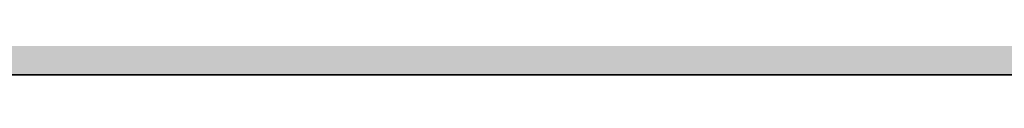
# Model space of a CAD drawing. Units: inches. Extents: x 2083 to 3317, y 1141 to 2115.
# Tile 127 of 256: x 3119.674 to 3123.979, y 1263.261 to 1263.355. Entities that reach past the tile are written whole.
import ezdxf

# ---------------------------------------------------------------- set-up
doc = ezdxf.new("R2010")
doc.units = ezdxf.units.IN
doc.layers.add('A-ANNO-DIMS', color=2, linetype='Continuous', lineweight=18)
doc.layers.add('A-WALL', color=7, linetype='Continuous', lineweight=35)
doc.layers.add('A-WALL-PATT', color=251, linetype='Continuous', lineweight=13, true_color=0x636466)
doc.styles.get("Standard").update_dxf_attribs({"font": 'arial.ttf'})
doc.dimstyles.new('ISO-25', dxfattribs={"dimtxt": 12, "dimasz": 12, "dimexe": 1.25, "dimexo": 0.625, "dimtad": 1, "dimlunit": 3, "dimtxsty": 'Standard', "dimcen": 2.5, "dimadec": 0, "dimazin": 0, "dimtfac": 1, "dimtmove": 0, "dimatfit": 3, "dimfxl": 1, "dimarcsym": 0})

# ---------------------------------------------------------------- blocks, each defined once
blk = doc.blocks.new('*D10')
at = {"layer": 'A-ANNO-DIMS', "color": 0, "lineweight": -2, "transparency": 16777216}
for p, q in [((2862.9598, 1262.6364), (2862.9598, 1201.3844)), ((3126.9598, 1262.6364), (3126.9598, 1201.3844)), ((2874.9598, 1202.6344), (3114.9598, 1202.6344))]:
    blk.add_line(p, q, dxfattribs=at)
at = {"layer": 'A-ANNO-DIMS', "color": 0, "transparency": 16777216}
for points in [[(2874.9598, 1204.6344), (2874.9598, 1200.6344), (2862.9598, 1202.6344)], [(3114.9598, 1204.6344), (3114.9598, 1200.6344), (3126.9598, 1202.6344)]]:
    blk.add_solid(points, dxfattribs=at)
at = {"layer": 'Defpoints', "color": 0, "transparency": 16777216}
for p in [(2862.9598, 1263.2614), (3126.9598, 1263.2614), (3126.9598, 1202.6344)]:
    blk.add_point(p, dxfattribs=at)
at = {"layer": 'A-ANNO-DIMS', "color": 0, "transparency": 16777216, "insert": (2994.9598, 1209.284), "char_height": 12, "attachment_point": 5}
blk.add_mtext("22'", dxfattribs=at)
blk = doc.blocks.new('*D26')
at = {"layer": 'A-ANNO-DIMS', "color": 0, "lineweight": -2, "transparency": 16777216}
for p, q in [((3088.9858, 1274.9151), (3088.9858, 1270.952)), ((3111.24, 1274.9151), (3111.24, 1270.952)), ((3076.9858, 1272.202), (2840.2624, 1272.202)), ((3111.24, 1272.202), (3088.9858, 1272.202)), ((3123.24, 1272.202), (3135.24, 1272.202))]:
    blk.add_line(p, q, dxfattribs=at)
at = {"layer": 'A-ANNO-DIMS', "color": 0, "transparency": 16777216}
for points in [[(3076.9858, 1274.202), (3076.9858, 1270.202), (3088.9858, 1272.202)], [(3123.24, 1274.202), (3123.24, 1270.202), (3111.24, 1272.202)]]:
    blk.add_solid(points, dxfattribs=at)
at = {"layer": 'Defpoints', "color": 0, "transparency": 16777216}
for p in [(3088.9858, 1275.5401), (3111.24, 1275.5401), (3088.9858, 1272.202)]:
    blk.add_point(p, dxfattribs=at)
at = {"layer": 'A-ANNO-DIMS', "color": 0, "transparency": 16777216, "insert": (2952.6241, 1279.0316), "char_height": 12, "attachment_point": 5}
blk.add_mtext('NIGHTSTAND 1\'-10 1/2" TYP.', dxfattribs=at)
blk = doc.blocks.new('*D27')
at = {"layer": 'A-ANNO-DIMS', "color": 0, "lineweight": -2, "transparency": 16777216}
for p, q in [((3114.5782, 1309.7943), (3114.5782, 1321.7943)), ((3111.865, 1297.7943), (3115.8282, 1297.7943)), ((3114.5782, 1297.7943), (3114.5782, 1275.5401)), ((3111.865, 1275.5401), (3115.8282, 1275.5401)), ((3114.5782, 1263.5401), (3114.5782, 1140.9886))]:
    blk.add_line(p, q, dxfattribs=at)
at = {"layer": 'A-ANNO-DIMS', "color": 0, "transparency": 16777216}
for points in [[(3112.5782, 1309.7943), (3116.5782, 1309.7943), (3114.5782, 1297.7943)], [(3112.5782, 1263.5401), (3116.5782, 1263.5401), (3114.5782, 1275.5401)]]:
    blk.add_solid(points, dxfattribs=at)
at = {"layer": 'Defpoints', "color": 0, "transparency": 16777216}
for p in [(3111.24, 1297.7943), (3111.24, 1275.5401), (3114.5782, 1275.5401)]:
    blk.add_point(p, dxfattribs=at)
at = {"layer": 'A-ANNO-DIMS', "color": 0, "transparency": 16777216, "insert": (3107.7485, 1196.2643), "char_height": 12, "attachment_point": 5, "rotation": 90}
blk.add_mtext('1\'-10 1/2" TYP.', dxfattribs=at)

msp = doc.modelspace()

# ---------------------------------------------------------------- hatches: boundary and pattern name
at = {"layer": 'A-WALL-PATT'}
h = msp.add_hatch(color=256, dxfattribs=at)
h.dxf.hatch_style = 1
h.paths.add_polyline_path([(3126.9598, 2020.7614), (2748.9598, 2020.7614), (2604.9598, 2020.7614), (2226.9598, 2020.7614), (2226.9598, 1702.7614), (2466.9598, 1702.7614), (2466.9598, 1582.7614), (2418.9598, 1582.7614), (2418.9598, 1477.7614), (2226.9598, 1477.7614), (2226.9598, 1263.2614), (2544.9598, 1263.2614), (2544.9598, 1411.7614), (2604.9598, 1411.7614), (2685.9598, 1411.7614), (2685.9598, 1420.7614), (2604.9598, 1420.7614), (2604.9598, 1573.7614), (2604.9598, 1702.7614), (2604.9598, 2011.7614), (2748.9598, 2011.7614), (2748.9598, 1702.7614), (2862.9598, 1702.7614), (2862.9598, 1621.7614), (2871.9598, 1621.7614), (2871.9598, 1702.7614), (2883.9598, 1702.7614), (2883.9598, 1706.9395, -0.026459), (2883.9598, 1711.7614), (2757.9598, 1711.7614), (2757.9598, 1807.7614), (2787.9598, 1807.7614), (2787.9598, 1812.2614), (2757.9598, 1812.2614), (2757.9598, 2011.7614), (2877.9598, 2011.7614), (2877.9598, 1812.2614), (2847.9598, 1812.2614), (2847.9598, 1807.7614), (2889.8357, 1807.7614), (2889.8357, 1812.2614), (2882.4598, 1812.2614), (2882.4598, 2011.7614), (3117.9598, 2011.7614), (3117.9598, 1812.2614), (2937.8357, 1812.2614), (2937.8357, 1807.7614), (2995.7098, 1807.7614), (2995.7098, 1796.1177), (3000.2098, 1796.1177), (3000.2098, 1807.7614), (3117.9598, 1807.7614), (3117.9598, 1711.7614), (3000.2098, 1711.7614), (3000.2098, 1760.1177), (2998.5727, 1760.1177, -0.020711), (2995.7098, 1760.1177), (2995.7098, 1711.7614), (2931.9598, 1711.7614), (2931.9598, 1702.7614), (3126.9598, 1702.7614)])
h.paths.add_polyline_path([(2471.4598, 2011.7614), (2471.4598, 1810.0114), (2462.7169, 1810.0114), (2462.7169, 1805.5114), (2505.9598, 1805.5114), (2505.9598, 1810.0114), (2475.9598, 1810.0114), (2475.9598, 2011.7614), (2595.9598, 2011.7614), (2595.9598, 1810.0114), (2565.9598, 1810.0114), (2565.9598, 1805.5114), (2595.9598, 1805.5114), (2595.9598, 1711.7614), (2235.9598, 1711.7614), (2235.9598, 1805.5114), (2353.7098, 1805.5114), (2353.7098, 1796.0542), (2358.2098, 1796.0542), (2358.2098, 1805.5114), (2414.7169, 1805.5114), (2414.7169, 1810.0114), (2235.9598, 1810.0114), (2235.9598, 2011.7614)], flags=16)
h.paths.add_polyline_path([(2270.2047, 1994.61), (2270.2047, 1970.61), (2246.2047, 1970.61), (2246.2047, 1994.61)], flags=0)
edge = h.paths.add_edge_path(flags=0)
edge.add_ellipse((2332.0274, 1899.7982), major_axis=(-3.043, 3.043), ratio=0.168252, start_angle=-161.3322, end_angle=-156.3071, ccw=False)
edge.add_ellipse((2333.082, 1898.7435), major_axis=(-1.0546, 1.0546), ratio=0.453532, start_angle=-123.371, end_angle=-94.1591)
edge = h.paths.add_edge_path(flags=0)
edge.add_ellipse((2332.0274, 1968.8763), major_axis=(3.043, 3.043), ratio=0.168252, start_angle=18.6678, end_angle=23.6929)
edge.add_spline(control_points=[(2332.9256, 1970.6911), (2332.2268, 1970.3361), (2330.8937, 1969.6589), (2328.4131, 1970.9321), (2327.2039, 1967.7487), (2324.7096, 1969.9556), (2322.5328, 1967.0124), (2320.0128, 1971.2958), (2317.6803, 1968.1578), (2316.0405, 1967.102), (2315.4269, 1966.8096)], knot_values=[0, 0, 0, 0, 2.267059, 4.324559, 6.685584, 8.878641, 11.121502, 14.300359, 17.755284, 19.732645, 19.732645, 19.732645, 19.732645], degree=3, periodic=0)
edge.add_ellipse((2332.0274, 1968.8763), major_axis=(3.043, 3.043), ratio=0.168252, start_angle=18.6678, end_angle=23.6929, ccw=False)
edge.add_ellipse((2333.082, 1969.9309), major_axis=(1.0546, 1.0546), ratio=0.453532, start_angle=56.629, end_angle=85.8409, ccw=False)
edge = h.paths.add_edge_path(flags=0)
edge.add_spline(control_points=[(2296.4283, 1967.9879), (2293.6278, 1965.3363), (2287.7036, 1959.7271), (2299.7439, 1949.9957), (2294.5326, 1935.6685), (2290.5732, 1920.6035), (2293.3941, 1909.9737), (2296.1854, 1904.9665)], knot_values=[0.099185, 0.099185, 0.099185, 0.099185, 0.345301, 0.619822, 0.982653, 1.386093, 1.810555, 1.810555, 1.810555, 1.810555], degree=3, periodic=0)
edge.add_spline(control_points=[(2296.1854, 1904.9665), (2297.3836, 1902.6193), (2298.001, 1901.9493), (2298.553, 1901.4682)], knot_values=[0.006246, 0.006246, 0.006246, 0.006246, 0.055476, 0.055476, 0.055476, 0.055476], degree=3, periodic=0)
edge.add_spline(control_points=[(2298.553, 1901.4682), (2297.2586, 1900.9232), (2295.2253, 1900.2321), (2293.0602, 1900.6142), (2292.1014, 1900.7884), (2292.0896, 1900.7906)], knot_values=[0.312835, 0.312835, 0.312835, 0.312835, 0.40178, 0.474987, 0.475903, 0.475903, 0.475903, 0.475903], degree=3, periodic=0)
edge.add_arc((2292.7936, 1904.6641), 3.937, 215.4209, 259.6982, ccw=False)
edge.add_spline(control_points=[(2289.5853, 1902.3823), (2289.4767, 1902.5351), (2289.3685, 1902.688), (2289.2609, 1902.8412)], knot_values=[0.102872, 0.102872, 0.102872, 0.102872, 0.116896, 0.116896, 0.116896, 0.116896], degree=3, periodic=0)
edge.add_spline(control_points=[(2289.2609, 1902.8412), (2288.6866, 1902.5502), (2287.64, 1902.0199), (2285.8813, 1901.874), (2283.853, 1901.5044), (2281.72, 1899.7105), (2278.467, 1899.4929), (2276.1571, 1901.8832), (2272.259, 1899.8041), (2267.7776, 1901.8432), (2262.2439, 1900.184), (2257.4149, 1901.7821), (2254.3184, 1900.7261), (2253.1783, 1900.3373)], knot_values=[0, 0, 0, 0, 1.907977, 3.477176, 5.261074, 7.972851, 11.680248, 13.717921, 16.939592, 22.789562, 27.502503, 33.595215, 37.145618, 37.145618, 37.145618, 37.145618], degree=3, periodic=0)
edge.add_line((2253.1783, 1900.3373), (2250.2442, 1902.8412))
edge.add_line((2250.2442, 1902.8412), (2250.2442, 1965.8333))
edge.add_line((2250.2442, 1965.8333), (2253.1783, 1968.3371))
edge.add_spline(control_points=[(2253.1783, 1968.3371), (2254.3184, 1967.9483), (2257.4149, 1966.8924), (2262.2439, 1968.4904), (2267.7776, 1966.8313), (2271.5267, 1968.5372), (2273.8759, 1967.8283), (2274.2067, 1967.7276)], knot_values=[0, 0, 0, 0, 0.09018, 0.244935, 0.364644, 0.513233, 0.537855, 0.537855, 0.537855, 0.537855], degree=3, periodic=0)
edge.add_arc((2274.3529, 1963.7933), 3.937, 72.0511, 92.1279, ccw=False)
edge.add_arc((2281.2969, 1985.23), 18.5963, 252.05113, 288.56572)
edge.add_arc((2292.3167, 1956.0289), 12.6461, 71.02679, 113.77822, ccw=False)
edge = h.paths.add_edge_path(flags=0)
edge.add_spline(control_points=[(2274.8994, 1951.8562), (2275.0662, 1951.6166), (2275.2327, 1951.3766), (2275.398, 1951.1359)], knot_values=[1.409916, 1.409916, 1.409916, 1.409916, 1.43159, 1.43159, 1.43159, 1.43159], degree=3, periodic=0)
edge.add_spline(control_points=[(2275.398, 1951.1359), (2275.7921, 1950.5619), (2276.1792, 1949.9838), (2276.5455, 1949.3971)], knot_values=[1.358238, 1.358238, 1.358238, 1.358238, 1.409916, 1.409916, 1.409916, 1.409916], degree=3, periodic=0)
edge.add_line((2276.5455, 1949.3971), (2277.4373, 1947.8622))
edge.add_spline(control_points=[(2277.4373, 1947.8622), (2276.3038, 1945.6731), (2274.6397, 1942.4269), (2274.6316, 1938.0939), (2272.7991, 1930.8515), (2274.3564, 1943.897), (2275.9477, 1947.9234), (2276.5455, 1949.3971)], knot_values=[0.005632, 0.005632, 0.005632, 0.005632, 0.186014, 0.266002, 0.357087, 0.59639, 0.739732, 0.739732, 0.739732, 0.739732], degree=3, periodic=0)
edge.add_spline(control_points=[(2276.5455, 1949.3971), (2276.1792, 1949.9838), (2275.7921, 1950.5619), (2275.398, 1951.1359)], knot_values=[1.358238, 1.358238, 1.358238, 1.358238, 1.409916, 1.409916, 1.409916, 1.409916], degree=3, periodic=0)
edge.add_spline(control_points=[(2275.398, 1951.1359), (2274.9425, 1950.0805), (2274.2078, 1948.0253), (2273.9346, 1944.8515), (2272.4685, 1937.6275), (2273.4662, 1945.6965), (2274.7006, 1951.0595), (2274.8994, 1951.8562)], knot_values=[0.104364, 0.104364, 0.104364, 0.104364, 0.189636, 0.269624, 0.36071, 0.600013, 0.644622, 0.644622, 0.644622, 0.644622], degree=3, periodic=0)
h.paths.add_polyline_path([(2269.1675, 1963.1276, -0.357527), (2268.1706, 1960.9764, -0.092561), (2268.1706, 1939.4363, -0.357527), (2269.1675, 1937.2851, -0.357527), (2267.0163, 1938.282, -0.164785), (2254.6856, 1938.282, -0.357527), (2252.5344, 1937.2851, -0.357527), (2253.5313, 1939.4363, -0.092561), (2253.5313, 1960.9764, -0.357527), (2252.5344, 1963.1276, -0.357527), (2254.6856, 1962.1307, -0.164785), (2267.0163, 1962.1307, -0.357527)], flags=0)
h.paths.add_polyline_path([(2248.8741, 1967.8018), (2248.8741, 1957.0277), (2249.4578, 1957.0277), (2249.4578, 1911.6468), (2248.8741, 1911.6468), (2248.8741, 1900.8727), (2246.5119, 1900.8727, 0.197327), (2244.1497, 1902.4569), (2244.1497, 1966.2176, 0.197327), (2246.5119, 1967.8018)], flags=0)
h.paths.add_polyline_path([(2269.1675, 1931.3893, -0.357527), (2268.1706, 1929.2381, -0.092561), (2268.1706, 1907.6981, -0.357527), (2269.1675, 1905.5469, -0.357527), (2267.0163, 1906.5438, -0.164785), (2254.6856, 1906.5438, -0.357527), (2252.5344, 1905.5469, -0.357527), (2253.5313, 1907.6981, -0.092561), (2253.5313, 1929.2381, -0.357527), (2252.5344, 1931.3893, -0.357527), (2254.6856, 1930.3925, -0.164785), (2267.0163, 1930.3925, -0.357527)], flags=0)
edge = h.paths.add_edge_path(flags=0)
edge.add_spline(control_points=[(2276.1969, 1906.7237), (2276.1681, 1909.0289), (2276.114, 1913.3719), (2270.5984, 1924.925), (2273.9052, 1919.0128), (2275.9217, 1916.2621), (2275.4746, 1912.4021), (2277.2579, 1910.3806), (2276.696, 1908.225), (2276.6462, 1906.813), (2276.6178, 1906.0084)], knot_values=[0, 0, 0, 0, 8.61026, 16.221274, 18.843057, 23.804898, 27.440828, 29.356102, 31.203478, 33.650687, 33.650687, 33.650687, 33.650687], degree=3, periodic=0)
edge.add_spline(control_points=[(2276.6178, 1906.0084), (2276.6233, 1905.6241), (2276.4977, 1904.6287), (2275.4418, 1903.8547), (2274.9373, 1903.0804), (2274.8591, 1902.8412)], knot_values=[0.156488, 0.156488, 0.156488, 0.156488, 0.184398, 0.231376, 0.250598, 0.250598, 0.250598, 0.250598], degree=3, periodic=0)
edge.add_line((2274.8591, 1902.8412), (2276.506, 1902.8412))
edge.add_spline(control_points=[(2276.506, 1902.8412), (2276.7883, 1903.0849), (2277.6651, 1904.1252), (2278.2495, 1904.3407), (2277.6539, 1908.5274), (2278.1557, 1906.2278), (2278.1005, 1905.2859), (2278.8467, 1904.069), (2277.8568, 1903.4149), (2277.8742, 1902.991), (2277.9036, 1902.8412)], knot_values=[0.059574, 0.059574, 0.059574, 0.059574, 0.080753, 0.103741, 0.16972, 0.176036, 0.207137, 0.240474, 0.262341, 0.27366, 0.27366, 0.27366, 0.27366], degree=3, periodic=0)
edge.add_line((2277.9036, 1902.8412), (2280.0298, 1902.8412))
edge.add_spline(control_points=[(2280.0298, 1902.8412), (2279.8882, 1903.0884), (2279.4993, 1903.9816), (2280.1523, 1905.9393), (2278.1036, 1909.6578), (2279.7624, 1907.1853), (2280.3279, 1904.8749), (2280.4851, 1903.4896), (2281.4633, 1903.2494), (2281.7583, 1902.9365), (2281.834, 1902.8412)], knot_values=[0.013856, 0.013856, 0.013856, 0.013856, 0.034874, 0.088867, 0.107879, 0.126738, 0.158714, 0.193757, 0.217487, 0.226722, 0.226722, 0.226722, 0.226722], degree=3, periodic=0)
edge.add_spline(control_points=[(2281.834, 1902.8412), (2281.7875, 1902.8267), (2281.647, 1902.783), (2281.3955, 1902.8595), (2281.0881, 1902.9852), (2280.7207, 1903.0609), (2280.3335, 1903.0257), (2280.1248, 1902.8989), (2280.0298, 1902.8412)], knot_values=[0, 0, 0, 0, 0.14413, 0.435517, 0.749276, 1.153046, 1.548371, 1.878348, 1.878348, 1.878348, 1.878348], degree=3, periodic=0)
edge.add_line((2280.0298, 1902.8412), (2277.9036, 1902.8412))
edge.add_spline(control_points=[(2277.9036, 1902.8412), (2277.8929, 1902.7959), (2277.8654, 1902.6796), (2277.6075, 1902.6875), (2277.2741, 1902.8007), (2276.8379, 1902.6198), (2276.5838, 1902.7893), (2276.506, 1902.8412)], knot_values=[0, 0, 0, 0, 0.127189, 0.326199, 0.628009, 1.24357, 1.515331, 1.515331, 1.515331, 1.515331], degree=3, periodic=0)
edge.add_line((2276.506, 1902.8412), (2274.8591, 1902.8412))
edge.add_spline(control_points=[(2274.8591, 1902.8412), (2274.8144, 1902.8986), (2274.7251, 1903.0134), (2274.4935, 1903.119), (2274.2443, 1902.9605), (2273.9371, 1903.1849), (2273.614, 1902.9831), (2273.4083, 1902.883), (2273.3223, 1902.8412)], knot_values=[0, 0, 0, 0, 0.21843, 0.436957, 0.687977, 0.990379, 1.398396, 1.69185, 1.69185, 1.69185, 1.69185], degree=3, periodic=0)
edge.add_spline(control_points=[(2273.3223, 1902.8412), (2273.6167, 1903.4457), (2274.274, 1904.5383), (2276.0272, 1904.5737), (2276.207, 1906.5836), (2276.1969, 1906.7237)], knot_values=[0.012227, 0.012227, 0.012227, 0.012227, 0.059472, 0.106218, 0.134458, 0.134458, 0.134458, 0.134458], degree=3, periodic=0)
h.paths.add_polyline_path([(2270.7761, 1897.7898), (2270.7761, 1873.7898), (2246.7761, 1873.7898), (2246.7761, 1897.7898)], flags=0)
h.paths.add_polyline_path([(2353.7098, 1760.0051), (2353.7098, 1760.0542), (2358.2098, 1760.0542, -0.033729)], flags=0)
h.paths.add_polyline_path([(2321.8191, 1737.5292), (2341.9953, 1737.5292, -0.414214), (2343.2033, 1736.3212), (2343.2033, 1721.0206, -0.414214), (2341.9953, 1719.8127), (2321.8191, 1719.8127, -0.414214), (2320.6112, 1721.0206), (2320.6112, 1736.3212, -0.414214)], flags=0)
h.paths.add_polyline_path([(2324.235, 1736.3212), (2339.5794, 1736.3212, -0.414214), (2341.9953, 1733.9053), (2341.9953, 1725.4497, -0.414214), (2339.5794, 1723.0338), (2333.6806, 1723.0338), (2333.8453, 1722.0455, -0.870646), (2335.4254, 1721.8259, -0.767327), (2333.9227, 1721.4232), (2331.291, 1721.4232, -0.767327), (2329.7883, 1721.8259, -0.870646), (2331.3684, 1722.0455), (2331.5331, 1723.0338), (2324.235, 1723.0338, -0.414214), (2321.8191, 1725.4497), (2321.8191, 1733.9053, -0.414214)], flags=0)
h.paths.add_polyline_path([(2570.4838, 1928.6154), (2589.6838, 1928.6154), (2590.1688, 1928.6154), (2590.1688, 1904.9934), (2570.4838, 1904.9934)], flags=0)
h.paths.add_polyline_path([(2574.4473, 1927.2638, -1), (2572.8288, 1927.2638, -1)], flags=0)
h.paths.add_polyline_path([(2573.0899, 1926.9409), (2573.925, 1927.776), (2574.1477, 1927.5533), (2573.3126, 1926.7182)], flags=0)
h.paths.add_polyline_path([(2578.7791, 1919.7296, -1), (2571.5917, 1919.7296, -1)], flags=0)
h.paths.add_polyline_path([(2578.3854, 1919.7296, -1), (2571.9854, 1919.7296, -1)], flags=0)
h.paths.add_polyline_path([(2331.5958, 1729.4762, -1), (2333.618, 1729.4762, -1)], flags=0)
h.paths.add_polyline_path([(2578.0342, 1927.2638, -1), (2576.4157, 1927.2638, -1)], flags=0)
h.paths.add_polyline_path([(2576.6889, 1927.5311), (2576.9116, 1927.7538), (2577.7467, 1926.9186), (2577.524, 1926.6959)], flags=0)
h.paths.add_polyline_path([(2578.1391, 1909.8595, -1), (2572.2317, 1909.8595, -1)], flags=0)
h.paths.add_polyline_path([(2577.7454, 1909.8595, -1), (2572.6254, 1909.8595, -1)], flags=0)
h.paths.add_polyline_path([(2583.7977, 1927.2638, -1), (2582.1792, 1927.2638, -1)], flags=0)
h.paths.add_polyline_path([(2582.7186, 1927.7538), (2583.5538, 1926.9186), (2583.3311, 1926.6959), (2582.4959, 1927.5311)], flags=0)
h.paths.add_polyline_path([(2582.4959, 1927.5311), (2582.7186, 1927.7538), (2583.5538, 1926.9186), (2583.3311, 1926.6959)], flags=0)
h.paths.add_polyline_path([(2587.7391, 1920.5296, -1), (2581.8317, 1920.5296, -1)], flags=0)
h.paths.add_polyline_path([(2587.3454, 1920.5296, -1), (2582.2254, 1920.5296, -1)], flags=0)
h.paths.add_polyline_path([(2587.3846, 1927.2638, -1), (2585.7661, 1927.2638, -1)], flags=0)
h.paths.add_polyline_path([(2586.082, 1926.9802), (2586.9172, 1927.8154), (2587.1399, 1927.5927), (2586.3047, 1926.7575)], flags=0)
h.paths.add_polyline_path([(2588.3791, 1910.6595, -1), (2581.1917, 1910.6595, -1)], flags=0)
h.paths.add_polyline_path([(2587.9854, 1910.6595, -1), (2581.5854, 1910.6595, -1)], flags=0)
h.paths.add_polyline_path([(2417.1677, 1729.4779), (2437.3439, 1729.4779, -0.414214), (2438.5519, 1728.2699), (2438.5519, 1712.9693, -0.414214), (2437.3439, 1711.7614), (2417.1677, 1711.7614, -0.414214), (2415.9598, 1712.9693), (2415.9598, 1728.2699, -0.414214)], flags=0)
h.paths.add_polyline_path([(2419.5836, 1728.2699), (2434.928, 1728.2699, -0.414214), (2437.3439, 1725.8541), (2437.3439, 1717.3984, -0.414214), (2434.928, 1714.9825), (2429.0292, 1714.9825), (2429.1939, 1713.9942, -0.870646), (2430.774, 1713.7746, -0.767327), (2429.2713, 1713.372), (2426.6396, 1713.372, -0.767327), (2425.1369, 1713.7746, -0.870646), (2426.717, 1713.9942), (2426.8817, 1714.9825), (2419.5836, 1714.9825, -0.414214), (2417.1677, 1717.3984), (2417.1677, 1725.8541, -0.414214)], flags=0)
h.paths.add_polyline_path([(2419.5836, 1728.2699), (2434.928, 1728.2699, -0.414214), (2437.3439, 1725.8541), (2437.3439, 1717.3984, -0.414214), (2434.928, 1714.9825), (2429.0292, 1714.9825), (2428.3581, 1719.009), (2427.5528, 1719.009), (2426.8817, 1714.9825), (2419.5836, 1714.9825, -0.414214), (2417.1677, 1717.3984), (2417.1677, 1725.8541, -0.414214)], flags=0)
h.paths.add_polyline_path([(2426.9444, 1721.4249, -1), (2428.9666, 1721.4249, -1)], flags=0)
h.paths.add_polyline_path([(2475.9598, 1702.7614), (2595.9598, 1702.7614), (2595.9598, 1582.7614), (2475.9598, 1582.7614)], flags=16)
h.paths.add_polyline_path([(2427.9598, 1573.7614), (2595.9598, 1573.7614), (2595.9598, 1468.7614), (2595.9598, 1420.7614), (2384.4598, 1420.7614), (2384.4598, 1468.7614), (2427.9598, 1468.7614)], flags=16)
h.paths.add_polyline_path([(2379.9598, 1468.7614), (2379.9598, 1420.7614), (2235.9598, 1420.7614), (2235.9598, 1468.7614)], flags=16)
h.paths.add_polyline_path([(2317.816, 1466.6958), (2337.9922, 1466.6958, -0.414214), (2339.2002, 1465.4878), (2339.2002, 1450.1872, -0.414214), (2337.9922, 1448.9792), (2317.816, 1448.9792, -0.414214), (2316.6081, 1450.1872), (2316.6081, 1465.4878, -0.414214)], flags=0)
h.paths.add_polyline_path([(2320.2319, 1465.4878), (2335.5763, 1465.4878, -0.414214), (2337.9922, 1463.0719), (2337.9922, 1454.6163, -0.414214), (2335.5763, 1452.2004), (2329.6775, 1452.2004), (2329.8422, 1451.212, -0.870646), (2331.4223, 1450.9925, -0.767327), (2329.9196, 1450.5898), (2327.2879, 1450.5898, -0.767327), (2325.7852, 1450.9925, -0.870646), (2327.3653, 1451.212), (2327.53, 1452.2004), (2320.2319, 1452.2004, -0.414214), (2317.816, 1454.6163), (2317.816, 1463.0719, -0.414214)], flags=0)
h.paths.add_polyline_path([(2320.2319, 1465.4878), (2335.5763, 1465.4878, -0.414214), (2337.9922, 1463.0719), (2337.9922, 1454.6163, -0.414214), (2335.5763, 1452.2004), (2329.6775, 1452.2004), (2329.0064, 1456.2269), (2328.2011, 1456.2269), (2327.53, 1452.2004), (2320.2319, 1452.2004, -0.414214), (2317.816, 1454.6163), (2317.816, 1463.0719, -0.414214)], flags=0)
h.paths.add_polyline_path([(2327.5926, 1458.6428, -1), (2329.6148, 1458.6428, -1)], flags=0)
h.paths.add_polyline_path([(2244.4117, 1433.3405), (2241.9209, 1433.3405, -0.414214), (2240.0179, 1435.2435), (2240.0179, 1440.9528, -0.414211), (2241.9209, 1442.8559), (2244.4117, 1442.8559, -1.976472)], flags=0)
h.paths.add_polyline_path([(2245.3569, 1434.3975, -0.414214), (2245.3569, 1441.7988, -2.144098)], flags=0)
h.paths.add_polyline_path([(2535.9598, 1416.2614), (2535.9598, 1272.2614), (2235.9598, 1272.2614), (2235.9598, 1416.2614)], flags=16)
h.paths.add_polyline_path([(2260.1196, 1384.2928), (2260.1196, 1362.0386), (2237.8654, 1362.0386), (2237.8654, 1384.2928)], flags=0)
edge = h.paths.add_edge_path(flags=0)
edge.add_line((2318.2518, 1362.0933), (2318.1458, 1362.001))
edge.add_ellipse((2317.4451, 1360.431), major_axis=(2.8216, 2.8216), ratio=0.168252, start_angle=18.6678, end_angle=20.9481, ccw=False)
edge.add_ellipse((2318.423, 1361.409), major_axis=(0.9779, 0.9779), ratio=0.453532, start_angle=56.629, end_angle=70.2262, ccw=False)
edge = h.paths.add_edge_path(flags=0)
edge.add_line((2319.1074, 1295.5711), (2319.015, 1295.6771))
edge.add_ellipse((2317.4451, 1296.3778), major_axis=(-2.8216, 2.8216), ratio=0.168252, start_angle=-161.3322, end_angle=-159.0519, ccw=False)
edge.add_ellipse((2318.423, 1295.3999), major_axis=(-0.9779, 0.9779), ratio=0.453532, start_angle=-123.371, end_angle=-109.7738)
edge = h.paths.add_edge_path(flags=0)
edge.add_spline(control_points=[(2284.2103, 1301.1702), (2284.5807, 1300.4447), (2284.8912, 1299.892), (2285.1596, 1299.461)], knot_values=[0.039066, 0.039066, 0.039066, 0.039066, 0.055476, 0.055476, 0.055476, 0.055476], degree=3, periodic=0)
edge.add_line((2285.1596, 1299.461), (2284.2103, 1301.1702))
edge = h.paths.add_edge_path(flags=0)
edge.add_line((2280.4125, 1297.298), (2283.37, 1297.0361))
edge.add_line((2283.37, 1297.0361), (2286.4057, 1297.9263))
edge.add_spline(control_points=[(2286.4057, 1297.9263), (2285.3055, 1297.4631), (2284.3448, 1297.1292), (2283.37, 1297.0361)], knot_values=[0.394369, 0.394369, 0.394369, 0.394369, 0.475903, 0.475903, 0.475903, 0.475903], degree=3, periodic=0)
edge.add_spline(control_points=[(2283.37, 1297.0361), (2283.2814, 1297.0277), (2282.3163, 1296.9573), (2281.3125, 1297.1345), (2280.4234, 1297.296), (2280.4125, 1297.298)], knot_values=[0.312835, 0.312835, 0.312835, 0.312835, 0.320246, 0.393453, 0.394369, 0.394369, 0.394369, 0.394369], degree=3, periodic=0)
edge = h.paths.add_edge_path(flags=0)
edge.add_line((2284.4356, 1359.6073), (2280.4463, 1355.328))
edge.add_line((2280.4463, 1355.328), (2279.58, 1351.0178))
edge.add_line((2279.58, 1351.0178), (2282.413, 1346.5804))
edge.add_spline(control_points=[(2282.413, 1346.5804), (2283.1533, 1345.5892), (2284.2529, 1344.0289), (2284.801, 1342.3872), (2284.9352, 1341.8055)], knot_values=[1.240098, 1.240098, 1.240098, 1.240098, 1.332892, 1.382712, 1.382712, 1.382712, 1.382712], degree=3, periodic=0)
edge.add_spline(control_points=[(2284.9352, 1341.8055), (2285.3191, 1340.1406), (2285.233, 1338.4092), (2284.9099, 1336.6541)], knot_values=[1.097484, 1.097484, 1.097484, 1.097484, 1.240098, 1.240098, 1.240098, 1.240098], degree=3, periodic=0)
edge.add_spline(control_points=[(2284.9099, 1336.6541), (2284.5868, 1334.899), (2284.0267, 1333.1203), (2283.4626, 1331.3606)], knot_values=[0.95487, 0.95487, 0.95487, 0.95487, 1.097484, 1.097484, 1.097484, 1.097484], degree=3, periodic=0)
edge.add_line((2283.4626, 1331.3606), (2281.8904, 1326.1534))
edge.add_line((2281.8904, 1326.1534), (2280.7563, 1321.0561))
edge.add_line((2280.7563, 1321.0561), (2280.2992, 1316.002))
edge.add_line((2280.2992, 1316.002), (2280.7159, 1310.9501))
edge.add_line((2280.7159, 1310.9501), (2282.0281, 1305.9721))
edge.add_line((2282.0281, 1305.9721), (2284.2103, 1301.1702))
edge.add_spline(control_points=[(2284.2103, 1301.1702), (2283.3407, 1302.7302), (2282.6119, 1304.3365), (2282.0281, 1305.9721)], knot_values=[0.099185, 0.099185, 0.099185, 0.099185, 0.241799, 0.241799, 0.241799, 0.241799], degree=3, periodic=0)
edge.add_spline(control_points=[(2282.0281, 1305.9721), (2281.4443, 1307.6078), (2281.0055, 1309.2728), (2280.7159, 1310.9501)], knot_values=[0.241799, 0.241799, 0.241799, 0.241799, 0.384413, 0.384413, 0.384413, 0.384413], degree=3, periodic=0)
edge.add_spline(control_points=[(2280.7159, 1310.9501), (2280.4332, 1312.5876), (2280.2894, 1314.277), (2280.2989, 1315.962), (2280.2992, 1316.002)], knot_values=[0.384413, 0.384413, 0.384413, 0.384413, 0.523647, 0.527028, 0.527028, 0.527028, 0.527028], degree=3, periodic=0)
edge.add_spline(control_points=[(2280.2992, 1316.002), (2280.3123, 1317.687), (2280.4779, 1319.3679), (2280.7563, 1321.0561)], knot_values=[0.527028, 0.527028, 0.527028, 0.527028, 0.669642, 0.669642, 0.669642, 0.669642], degree=3, periodic=0)
edge.add_spline(control_points=[(2280.7563, 1321.0561), (2281.0346, 1322.7443), (2281.4259, 1324.4396), (2281.8904, 1326.1534)], knot_values=[0.669642, 0.669642, 0.669642, 0.669642, 0.812256, 0.812256, 0.812256, 0.812256], degree=3, periodic=0)
edge.add_spline(control_points=[(2281.8904, 1326.1534), (2282.2644, 1327.5333), (2282.7879, 1329.2618), (2283.3528, 1331.0178), (2283.4626, 1331.3606)], knot_values=[0.812256, 0.812256, 0.812256, 0.812256, 0.927087, 0.95487, 0.95487, 0.95487, 0.95487], degree=3, periodic=0)
edge.add_line((2283.4626, 1331.3606), (2284.9099, 1336.6541))
edge.add_line((2284.9099, 1336.6541), (2284.9352, 1341.8055))
edge.add_line((2284.9352, 1341.8055), (2282.413, 1346.5804))
edge.add_spline(control_points=[(2282.413, 1346.5804), (2281.2751, 1348.1038), (2280.0784, 1349.5703), (2279.58, 1351.0178)], knot_values=[1.382712, 1.382712, 1.382712, 1.382712, 1.525326, 1.525326, 1.525326, 1.525326], degree=3, periodic=0)
edge.add_spline(control_points=[(2279.58, 1351.0178), (2279.4433, 1351.4147), (2279.1363, 1352.8569), (2279.7352, 1354.2904), (2280.4463, 1355.328)], knot_values=[1.525326, 1.525326, 1.525326, 1.525326, 1.564439, 1.667941, 1.667941, 1.667941, 1.667941], degree=3, periodic=0)
edge.add_spline(control_points=[(2280.4463, 1355.328), (2281.4261, 1356.7578), (2282.9308, 1358.1826), (2284.4356, 1359.6073)], knot_values=[1.667941, 1.667941, 1.667941, 1.667941, 1.810555, 1.810555, 1.810555, 1.810555], degree=3, periodic=0)
edge.add_arc((2280.6231, 1348.5182), 11.7262, 71.02679, 113.77822)
edge.add_arc((2270.4049, 1375.5952), 17.2436, 252.05113, 288.56572, ccw=False)
edge.add_arc((2263.966, 1355.7178), 3.6506, 72.0511, 92.1279)
edge.add_arc((2263.966, 1355.7178), 3.6506, 92.1279, 177.9851)
edge.add_spline(control_points=[(2260.3176, 1355.8462), (2260.2604, 1354.2207), (2260.5513, 1350.1865), (2262.9993, 1346.7663), (2264.4727, 1344.649)], knot_values=[1.43159, 1.43159, 1.43159, 1.43159, 1.564144, 1.770695, 1.770695, 1.770695, 1.770695], degree=3, periodic=0)
edge.add_line((2264.4727, 1344.649), (2264.9356, 1343.9825))
edge.add_spline(control_points=[(2263.801, 1340.2481), (2263.8432, 1340.5141), (2264.0672, 1341.7565), (2264.5127, 1343.0025), (2264.935, 1343.9811)], knot_values=[0.53657, 0.53657, 0.53657, 0.53657, 0.559349, 0.644622, 0.644622, 0.644622, 0.644622], degree=3, periodic=0)
edge.add_spline(control_points=[(2264.935, 1343.9811), (2265.1178, 1343.715), (2265.2989, 1343.4479), (2265.4768, 1343.1794)], knot_values=[1.384077, 1.384077, 1.384077, 1.384077, 1.409916, 1.409916, 1.409916, 1.409916], degree=3, periodic=0)
edge.add_spline(control_points=[(2265.4768, 1343.1794), (2265.6546, 1342.9108), (2265.8293, 1342.6408), (2265.9991, 1342.3688)], knot_values=[1.358238, 1.358238, 1.358238, 1.358238, 1.384077, 1.384077, 1.384077, 1.384077], degree=3, periodic=0)
edge.add_line((2265.9991, 1342.3688), (2266.826, 1340.9455))
edge.add_spline(control_points=[(2266.826, 1340.9455), (2268.8944, 1337.0897), (2271.3982, 1325.843), (2270.5162, 1310.5686), (2275.9194, 1301.8606), (2277.7895, 1299.1994)], knot_values=[0.116896, 0.116896, 0.116896, 0.116896, 0.472987, 1.050969, 1.313793, 1.313793, 1.313793, 1.313793], degree=3, periodic=0)
edge.add_spline(control_points=[(2277.7895, 1299.1994), (2277.8394, 1299.1285), (2277.8894, 1299.0575), (2277.9396, 1298.9866)], knot_values=[0.109884, 0.109884, 0.109884, 0.109884, 0.116896, 0.116896, 0.116896, 0.116896], degree=3, periodic=0)
edge.add_line((2277.9396, 1298.9866), (2277.7888, 1299.1991))
edge.add_spline(control_points=[(2277.7888, 1299.1991), (2277.2566, 1298.9294), (2276.2864, 1298.4379), (2275.0394, 1298.3344), (2274.3833, 1298.2389), (2274.2153, 1298.2093)], knot_values=[33.12187, 33.12187, 33.12187, 33.12187, 35.029056, 36.598255, 37.144827, 37.144827, 37.144827, 37.144827], degree=3, periodic=0)
edge.add_line((2274.2153, 1298.2093), (2273.0731, 1297.893))
edge.add_spline(control_points=[(2273.0731, 1297.893), (2272.3229, 1297.5798), (2271.0392, 1296.5105), (2269.2484, 1296.2261), (2268.4231, 1296.3747)], knot_values=[26.532584, 26.532584, 26.532584, 26.532584, 29.198919, 31.839101, 31.839101, 31.839101, 31.839101], degree=3, periodic=0)
edge.add_line((2268.4231, 1296.3747), (2263.8785, 1297.4575))
edge.add_spline(control_points=[(2263.8785, 1297.4575), (2263.5561, 1297.3594), (2261.8603, 1296.8387), (2260.2388, 1297.2824), (2258.9335, 1297.5165)], knot_values=[15.919551, 15.919551, 15.919551, 15.919551, 16.939592, 21.226067, 21.226067, 21.226067, 21.226067], degree=3, periodic=0)
edge.add_line((2258.9335, 1297.5165), (2254.0552, 1297.329))
edge.add_spline(control_points=[(2254.0552, 1297.329), (2253.7555, 1297.2958), (2252.1137, 1297.1652), (2250.4619, 1297.5442), (2249.1297, 1297.6679)], knot_values=[5.306517, 5.306517, 5.306517, 5.306517, 6.276435, 10.613034, 10.613034, 10.613034, 10.613034], degree=3, periodic=0)
edge.add_line((2249.1297, 1297.6679), (2244.3316, 1296.8778))
edge.add_line((2244.3316, 1296.8778), (2241.611, 1299.1994))
edge.add_line((2241.611, 1299.1994), (2241.611, 1357.6094))
edge.add_line((2241.611, 1357.6094), (2244.3316, 1359.9311))
edge.add_line((2244.3316, 1359.9311), (2252.7288, 1359.5427))
edge.add_spline(control_points=[(2252.7288, 1359.5427), (2252.8709, 1359.5464), (2253.3057, 1359.5482), (2253.7398, 1359.5143), (2254.0317, 1359.4824)], knot_values=[0.233291, 0.233291, 0.233291, 0.233291, 0.244935, 0.268927, 0.268927, 0.268927, 0.268927], degree=3, periodic=0)
edge.add_line((2254.0317, 1359.4824), (2259.5872, 1359.4164))
edge.add_spline(control_points=[(2259.5872, 1359.4164), (2260.6771, 1359.6285), (2262.0732, 1359.897), (2263.5237, 1359.4593), (2263.8304, 1359.366)], knot_values=[0.422516, 0.422516, 0.422516, 0.422516, 0.513233, 0.537855, 0.537855, 0.537855, 0.537855], degree=3, periodic=0)
edge.add_arc((2263.966, 1355.7178), 3.6506, 72.0511, 92.1279, ccw=False)
edge.add_arc((2270.4049, 1375.5952), 17.2436, 252.05113, 288.56572)
edge.add_arc((2280.6231, 1348.5182), 11.7262, 71.02679, 113.77822, ccw=False)
h.paths.add_polyline_path([(2240.3405, 1359.4347), (2240.3405, 1349.4444), (2240.8818, 1349.4444), (2240.8818, 1307.3645), (2240.3405, 1307.3645), (2240.3405, 1297.3741), (2238.1502, 1297.3741, 0.197327), (2235.9598, 1298.8431), (2235.9598, 1357.9657, 0.197327), (2238.1502, 1359.4347)], flags=0)
h.paths.add_polyline_path([(2259.1578, 1355.1005, -0.357527), (2258.2334, 1353.1058, -0.092561), (2258.2334, 1333.1326, -0.357527), (2259.1578, 1331.1379, -0.357527), (2257.1631, 1332.0622, -0.164785), (2245.7293, 1332.0622, -0.357527), (2243.7346, 1331.1379, -0.357527), (2244.6589, 1333.1326, -0.092561), (2244.6589, 1353.1058, -0.357527), (2243.7346, 1355.1005, -0.357527), (2245.7293, 1354.1761, -0.164785), (2257.1631, 1354.1761, -0.357527)], flags=0)
edge = h.paths.add_edge_path(flags=0)
edge.add_line((2265.9991, 1342.3688), (2266.826, 1340.9455))
edge.add_line((2266.826, 1340.9455), (2265.3076, 1337.8141))
edge.add_line((2265.3076, 1337.8141), (2264.3582, 1334.6529))
edge.add_line((2264.3582, 1334.6529), (2264.262, 1333.7997))
edge.add_spline(control_points=[(2264.262, 1333.7997), (2264.2084, 1333.1871), (2264.1621, 1332.3655), (2264.0071, 1331.4139), (2263.969, 1331.2018)], knot_values=[0.464444, 0.464444, 0.464444, 0.464444, 0.516691, 0.531608, 0.531608, 0.531608, 0.531608], degree=3, periodic=0)
edge.add_spline(control_points=[(2263.969, 1331.2018), (2263.7745, 1330.1189), (2263.4244, 1328.7908), (2263.2574, 1328.5307), (2263.234, 1328.5146)], knot_values=[0.372682, 0.372682, 0.372682, 0.372682, 0.44885, 0.464444, 0.464444, 0.464444, 0.464444], degree=3, periodic=0)
edge.add_spline(control_points=[(2263.234, 1328.5146), (2263.0964, 1328.4202), (2263.1312, 1329.3015), (2263.275, 1330.6157)], knot_values=[0.280919, 0.280919, 0.280919, 0.280919, 0.372682, 0.372682, 0.372682, 0.372682], degree=3, periodic=0)
edge.add_spline(control_points=[(2263.275, 1330.6157), (2263.4187, 1331.93), (2263.6715, 1333.6773), (2263.9699, 1335.315)], knot_values=[0.189157, 0.189157, 0.189157, 0.189157, 0.280919, 0.280919, 0.280919, 0.280919], degree=3, periodic=0)
edge.add_spline(control_points=[(2263.9699, 1335.315), (2264.1005, 1336.0322), (2264.4188, 1337.6219), (2264.7548, 1338.8644), (2264.9474, 1339.4911)], knot_values=[0.097394, 0.097394, 0.097394, 0.097394, 0.137578, 0.189157, 0.189157, 0.189157, 0.189157], degree=3, periodic=0)
edge.add_spline(control_points=[(2264.9474, 1339.4911), (2265.29, 1340.6061), (2265.6442, 1341.494), (2265.9991, 1342.3688)], knot_values=[0.005632, 0.005632, 0.005632, 0.005632, 0.097394, 0.097394, 0.097394, 0.097394], degree=3, periodic=0)
h.paths.add_polyline_path([(2259.1578, 1325.671, -0.357527), (2258.2334, 1323.6763, -0.092561), (2258.2334, 1303.7031, -0.357527), (2259.1578, 1301.7084, -0.357527), (2257.1631, 1302.6327, -0.164785), (2245.7293, 1302.6327, -0.357527), (2243.7346, 1301.7084, -0.357527), (2244.6589, 1303.7031, -0.092561), (2244.6589, 1323.6763, -0.357527), (2243.7346, 1325.671, -0.357527), (2245.7293, 1324.7466, -0.164785), (2257.1631, 1324.7466, -0.357527)], flags=0)
edge = h.paths.add_edge_path(flags=0)
edge.add_spline(control_points=[(2261.7089, 1317.3114), (2261.6795, 1317.4176), (2261.7619, 1317.3885), (2262.4907, 1316.0899), (2262.9622, 1315.3009)], knot_values=[14.955861, 14.955861, 14.955861, 14.955861, 16.221274, 18.694826, 18.694826, 18.694826, 18.694826], degree=3, periodic=0)
edge.add_spline(control_points=[(2262.9622, 1315.3009), (2262.9904, 1315.2536), (2263.7021, 1314.0674), (2264.349, 1313.1272), (2264.7301, 1312.1642)], knot_values=[18.694826, 18.694826, 18.694826, 18.694826, 18.843057, 22.433791, 22.433791, 22.433791, 22.433791], degree=3, periodic=0)
edge.add_spline(control_points=[(2264.7301, 1312.1642), (2264.8756, 1311.7964), (2265.1769, 1310.7698), (2265.1431, 1309.5593), (2265.2477, 1308.8242)], knot_values=[22.433791, 22.433791, 22.433791, 22.433791, 23.804898, 26.172756, 26.172756, 26.172756, 26.172756], degree=3, periodic=0)
edge.add_line((2265.2477, 1308.8242), (2265.8508, 1307.1719))
edge.add_spline(control_points=[(2265.8508, 1307.1719), (2266.065, 1306.8217), (2266.3844, 1306.3322), (2266.4244, 1305.7805), (2266.4204, 1305.6112)], knot_values=[28.062562, 28.062562, 28.062562, 28.062562, 29.356102, 29.911721, 29.911721, 29.911721, 29.911721], degree=3, periodic=0)
edge.add_spline(control_points=[(2266.4204, 1305.6112), (2266.4161, 1305.4326), (2266.394, 1305.25), (2266.3648, 1305.0659)], knot_values=[29.911721, 29.911721, 29.911721, 29.911721, 30.497837, 30.497837, 30.497837, 30.497837], degree=3, periodic=0)
edge.add_line((2266.3648, 1305.0659), (2266.0662, 1302.1363))
edge.add_spline(control_points=[(2266.0662, 1302.1363), (2266.0712, 1301.78), (2265.9981, 1301.2), (2265.6633, 1300.759), (2265.5089, 1300.5859)], knot_values=[0.156488, 0.156488, 0.156488, 0.156488, 0.184398, 0.203543, 0.203543, 0.203543, 0.203543], degree=3, periodic=0)
edge.add_line((2265.5089, 1300.5859), (2264.4353, 1299.1994))
edge.add_line((2264.4353, 1299.1994), (2265.9624, 1299.1994))
edge.add_line((2265.9624, 1299.1994), (2267.336, 1301.1753))
edge.add_line((2267.336, 1301.1753), (2267.3117, 1301.9862))
edge.add_spline(control_points=[(2267.3117, 1301.9862), (2267.2611, 1302.8624), (2267.1602, 1303.7371), (2267.2715, 1303.3259)], knot_values=[0.126229, 0.126229, 0.126229, 0.126229, 0.166617, 0.166617, 0.166617, 0.166617], degree=3, periodic=0)
edge.add_spline(control_points=[(2267.2715, 1303.3259), (2267.28, 1303.2943), (2267.3098, 1303.1754), (2267.3735, 1302.8836), (2267.4061, 1302.6828), (2267.4179, 1302.601)], knot_values=[0.166617, 0.166617, 0.166617, 0.166617, 0.16972, 0.176036, 0.180765, 0.180765, 0.180765, 0.180765], degree=3, periodic=0)
edge.add_spline(control_points=[(2267.7439, 1300.9875), (2267.6876, 1301.1509), (2267.4805, 1301.6567), (2267.4838, 1302.1448), (2267.4179, 1302.601)], knot_values=[0.180765, 0.180765, 0.180765, 0.180765, 0.193767, 0.220139, 0.220139, 0.220139, 0.220139], degree=3, periodic=0)
edge.add_line((2267.4179, 1302.601), (2267.7439, 1300.9875))
edge.add_spline(control_points=[(2267.7439, 1300.9875), (2267.832, 1300.7319), (2267.932, 1300.3099), (2267.5548, 1299.9745), (2267.4294, 1299.8292)], knot_values=[0.220139, 0.220139, 0.220139, 0.220139, 0.240474, 0.25489, 0.25489, 0.25489, 0.25489], degree=3, periodic=0)
edge.add_line((2267.4294, 1299.8292), (2267.2584, 1299.1994))
edge.add_line((2267.2584, 1299.1994), (2269.23, 1299.1994))
edge.add_spline(control_points=[(2269.23, 1299.1994), (2269.0987, 1299.4287), (2268.8428, 1300.0163), (2269.0116, 1300.9159), (2268.9468, 1301.6607)], knot_values=[0.013856, 0.013856, 0.013856, 0.013856, 0.034874, 0.067073, 0.067073, 0.067073, 0.067073], degree=3, periodic=0)
edge.add_line((2268.9468, 1301.6607), (2268.4316, 1303.6031))
edge.add_spline(control_points=[(2268.4316, 1303.6031), (2268.1756, 1304.1924), (2267.5962, 1305.2513), (2268.0407, 1304.6232), (2268.2514, 1304.2824)], knot_values=[0.090155, 0.090155, 0.090155, 0.090155, 0.107879, 0.120289, 0.120289, 0.120289, 0.120289], degree=3, periodic=0)
edge.add_spline(control_points=[(2268.2514, 1304.2824), (2268.3609, 1304.1053), (2269.0578, 1302.918), (2269.3827, 1301.5904), (2269.5214, 1300.7759), (2269.5752, 1300.5558)], knot_values=[0.120289, 0.120289, 0.120289, 0.120289, 0.126738, 0.158714, 0.173506, 0.173506, 0.173506, 0.173506], degree=3, periodic=0)
edge.add_line((2269.5752, 1300.5558), (2270.6858, 1299.4213))
edge.add_spline(control_points=[(2270.6858, 1299.4213), (2270.7672, 1299.3573), (2270.8379, 1299.2814), (2270.9029, 1299.1994)], knot_values=[0.21816, 0.21816, 0.21816, 0.21816, 0.226722, 0.226722, 0.226722, 0.226722], degree=3, periodic=0)
edge.add_line((2270.9372, 1299.1929), (2270.9029, 1299.1994))
edge.add_spline(control_points=[(2270.9029, 1299.1994), (2270.8598, 1299.186), (2270.7295, 1299.1455), (2270.4963, 1299.2164), (2270.2717, 1299.3083), (2270.121, 1299.348), (2270.0633, 1299.3596)], knot_values=[0.939174, 0.939174, 0.939174, 0.939174, 1.083304, 1.374691, 1.68845, 1.878348, 1.878348, 1.878348, 1.878348], degree=3, periodic=0)
edge.add_line((2270.0633, 1299.3596), (2269.23, 1299.1994))
edge.add_line((2269.23, 1299.1994), (2267.2584, 1299.1994))
edge.add_spline(control_points=[(2267.2584, 1299.1994), (2267.2484, 1299.1574), (2267.223, 1299.0497), (2266.9838, 1299.0569), (2266.8092, 1299.1162), (2266.6769, 1299.1091), (2266.6365, 1299.1048)], knot_values=[0.757665, 0.757665, 0.757665, 0.757665, 0.884854, 1.083864, 1.385675, 1.515331, 1.515331, 1.515331, 1.515331], degree=3, periodic=0)
edge.add_spline(control_points=[(2266.6365, 1299.1048), (2266.4852, 1299.0888), (2266.2358, 1299.0171), (2266.0346, 1299.1513), (2265.9624, 1299.1994)], knot_values=[0, 0, 0, 0, 0.485905, 0.757665, 0.757665, 0.757665, 0.757665], degree=3, periodic=0)
edge.add_line((2265.9624, 1299.1994), (2264.4353, 1299.1994))
edge.add_line((2264.4353, 1299.1994), (2263.8584, 1299.3671))
edge.add_spline(control_points=[(2263.8584, 1299.3671), (2263.8189, 1299.3709), (2263.7795, 1299.3857), (2263.7401, 1299.4015)], knot_values=[0.845925, 0.845925, 0.845925, 0.845925, 0.978627, 0.978627, 0.978627, 0.978627], degree=3, periodic=0)
edge.add_line((2263.7218, 1299.3964), (2263.0103, 1299.1994))
edge.add_spline(control_points=[(2263.0103, 1299.1994), (2263.2458, 1299.6829), (2263.506, 1300.1281), (2263.8735, 1300.408)], knot_values=[0.012227, 0.012227, 0.012227, 0.012227, 0.052971, 0.052971, 0.052971, 0.052971], degree=3, periodic=0)
edge.add_spline(control_points=[(2263.8735, 1300.408), (2263.9321, 1300.4527), (2264.0842, 1300.553), (2264.2552, 1300.6242), (2264.3597, 1300.6647)], knot_values=[0.052971, 0.052971, 0.052971, 0.052971, 0.059472, 0.069086, 0.069086, 0.069086, 0.069086], degree=3, periodic=0)
edge.add_line((2264.3597, 1300.6647), (2265.1419, 1301.0778))
edge.add_line((2265.1419, 1301.0778), (2265.6758, 1302.7996))
edge.add_line((2265.6758, 1302.7996), (2265.5407, 1305.7041))
edge.add_line((2265.5407, 1305.7041), (2264.8031, 1309.3277))
edge.add_line((2264.8031, 1309.3277), (2263.0405, 1314.0918))
edge.add_spline(control_points=[(2263.0405, 1314.0918), (2262.3836, 1315.6714), (2261.796, 1316.9977), (2261.7089, 1317.3114)], knot_values=[11.216896, 11.216896, 11.216896, 11.216896, 14.955861, 14.955861, 14.955861, 14.955861], degree=3, periodic=0)
h.paths.add_polyline_path([(2871.9598, 1416.2614), (2895.91, 1416.2614), (2895.91, 1420.7614), (2871.9598, 1420.7614), (2871.9598, 1501.7614), (2862.9598, 1501.7614), (2862.9598, 1420.7614), (2805.9598, 1420.7614), (2805.9598, 1411.7614), (2862.9598, 1411.7614), (2862.9598, 1263.2614), (3126.9598, 1263.2614), (3126.9598, 1411.7614), (3126.9598, 1486.7614), (2943.9598, 1486.7614), (2943.9598, 1477.7614), (2967.8603, 1477.7614), (2967.8603, 1420.7614), (2943.91, 1420.7614), (2943.91, 1416.2614), (3117.9598, 1416.2614), (3117.9598, 1420.7614), (2972.3603, 1420.7614), (2972.3603, 1477.7614), (3117.9598, 1477.7614), (3117.9598, 1420.7614), (3117.9598, 1272.2614), (2871.9598, 1272.2614)], flags=0)
h.paths.add_polyline_path([(2457.1256, 1485.9425), (2527.6027, 1485.9425), (2527.6027, 1537.6357), (2457.1256, 1537.6357)], flags=8)
h.paths.add_polyline_path([(2481.0051, 1609.9818), (2590.7658, 1609.9818), (2590.7658, 1682.0034), (2481.0051, 1682.0034)], flags=8)
h.paths.add_polyline_path([(2483.085, 1729.1268), (2553.562, 1729.1268), (2553.562, 1780.82), (2483.085, 1780.82)], flags=8)
h = msp.add_hatch(color=256, dxfattribs=at)
h.dxf.hatch_style = 1
h.paths.add_polyline_path([(3126.9598, 1486.7614), (2943.9598, 1486.7614), (2943.9598, 1477.7614), (2967.8603, 1477.7614), (2967.8603, 1420.7614), (2943.91, 1420.7614), (2943.91, 1416.2614), (3117.9598, 1416.2614), (3117.9598, 1420.7614), (2972.3603, 1420.7614), (2972.3603, 1477.7614), (3117.9598, 1477.7614), (3117.9598, 1420.7614), (3117.9598, 1272.2614), (2871.9598, 1272.2614), (2871.9598, 1416.2614), (2895.91, 1416.2614), (2895.91, 1420.7614), (2871.9598, 1420.7614), (2871.9598, 1501.7614), (2862.9598, 1501.7614), (2862.9598, 1420.7614), (2805.9598, 1420.7614), (2805.9598, 1411.7614), (2862.9598, 1411.7614), (2862.9598, 1263.2614), (3126.9598, 1263.2614), (3126.9598, 1411.7614)])

# ---------------------------------------------------------------- linework, layer by layer
at = {"layer": 'A-WALL'}
msp.add_line((2544.9598, 1263.2614), (3126.9598, 1263.2614), dxfattribs=at)

# ---------------------------------------------------------------- dimensions: what is measured, and where the dimension line sits
at = {"layer": 'A-ANNO-DIMS'}
for base, p1, p2, angle, text, picture, middle in [((3114.5782, 1275.5401), (3111.24, 1297.7943), (3111.24, 1275.5401), 270, '<> TYP.', '*D27', (3107.7485, 1196.2643)), ((3088.9858, 1272.202), (3111.24, 1275.5401), (3088.9858, 1275.5401), 180, 'NIGHTSTAND <> TYP.', '*D26', (2952.6241, 1279.0316))]:
    dim = msp.add_linear_dim(base=base, p1=p1, p2=p2, angle=angle, text=text, dimstyle='ISO-25', override={"dimdec": 1, "dimlfac": 1, "dimrnd": 0, "dimzin": 1, "dimdsep": 46, "dimlunit": 4, "dimfrac": 2}, dxfattribs=at)
    dim.commit()
    dim.dimension.update_dxf_attribs({"geometry": picture, "text_midpoint": middle})
dim = msp.add_linear_dim(base=(3126.9598, 1202.6344), p1=(2862.9598, 1263.2614), p2=(3126.9598, 1263.2614), dimstyle='ISO-25', override={"dimclrd": 0, "dimclre": 0, "dimclrt": 0}, dxfattribs=at)
dim.commit()
dim.dimension.update_dxf_attribs({"geometry": '*D10', "text_midpoint": (2994.9598, 1209.284)})

doc.saveas('drawing.dxf')
